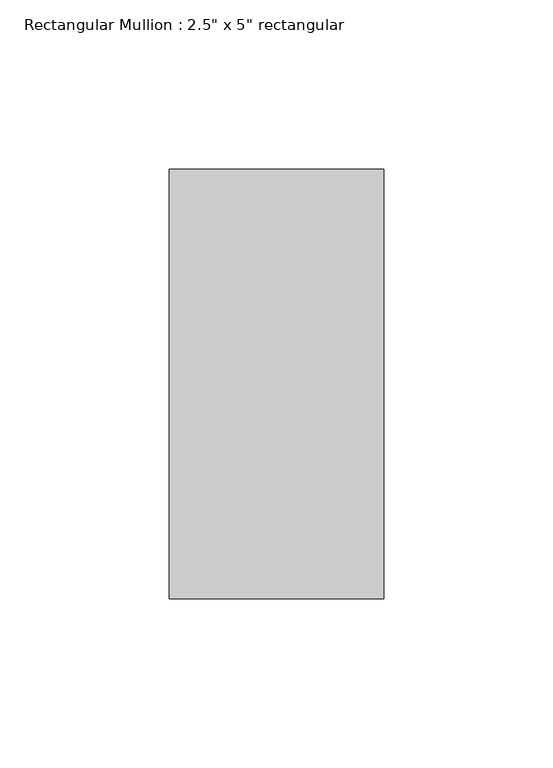
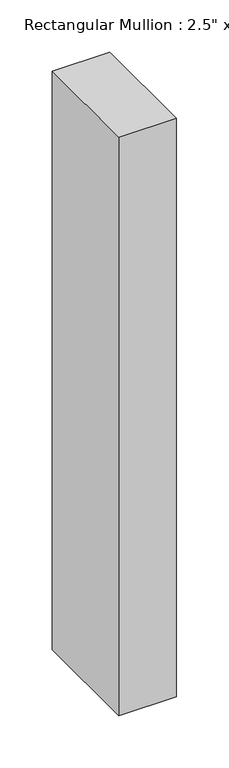
"""IFC4 building model written with IfcOpenShell, lengths in millimetres: member geometry."""

from ifc_helpers import new_model, si_unit, frame, origin, place, context, project, spatial, polyline, outline, extrude, source, transform, mapped, element, save


def member_0a83a24a(model_context):
    return source(origin(), model_context, "Body", "SweptSolid", [
        extrude(outline(polyline([(0.0, 63.5), (0.0, -63.5), (-63.5, -63.5), (-63.5, 63.5), (0.0, 63.5)])), frame((0.0, 0.0, -674.5371805), z_axis=(0.0, 0.0, 1.0), x_axis=(1.0, 0.0, 0.0)), (0.0, 0.0, 1.0), 674.5371805),
    ])


if __name__ == "__main__":
    model = new_model("IFC4")
    model_context = context("Model", 3, world=origin())
    ifc_project = project(units=[si_unit("LENGTHUNIT", "METRE", prefix="MILLI")], contexts=[model_context])
    site = spatial("IfcSite", under=ifc_project)
    building = spatial("IfcBuilding", under=site)
    placement = place(None, origin())
    member_shape = member_0a83a24a(model_context)
    element("IfcMember", 1, ObjectType="Rectangular Mullion : 2.5\" x 5\" rectangular", at=placement, inside=building, context=model_context, shape_type="MappedRepresentation", body=[
        mapped(member_shape, transform((0.0, 0.0, 0.0), x_axis=(1.0, 0.0, 0.0), y_axis=(0.0, 1.0, 0.0), z_axis=(0.0, 0.0, 1.0))),
    ])
    save(model, "model.ifc")

# Revit data of these elements
# Type "Rectangular Mullion : 2.5\" x 5\" rectangular"
#   built-in parameter 1007304 = 0.416667 (stored number, unit not read)
#   built-in parameter 1007301 = 0.104167 (stored number, unit not read)
#   built-in parameter 1007300 = 0.104167 (stored number, unit not read)
# Element 1 (IfcMember, "Rectangular Mullion : 2.5\" x 5\" rectangular")
#   Materials on its faces: "Aluminum"
# Materials
#   "Aluminum": class "Metal", colour RGB 247 247 247, transparency 0, Description = "Aluminum 6061", Cost = 0
